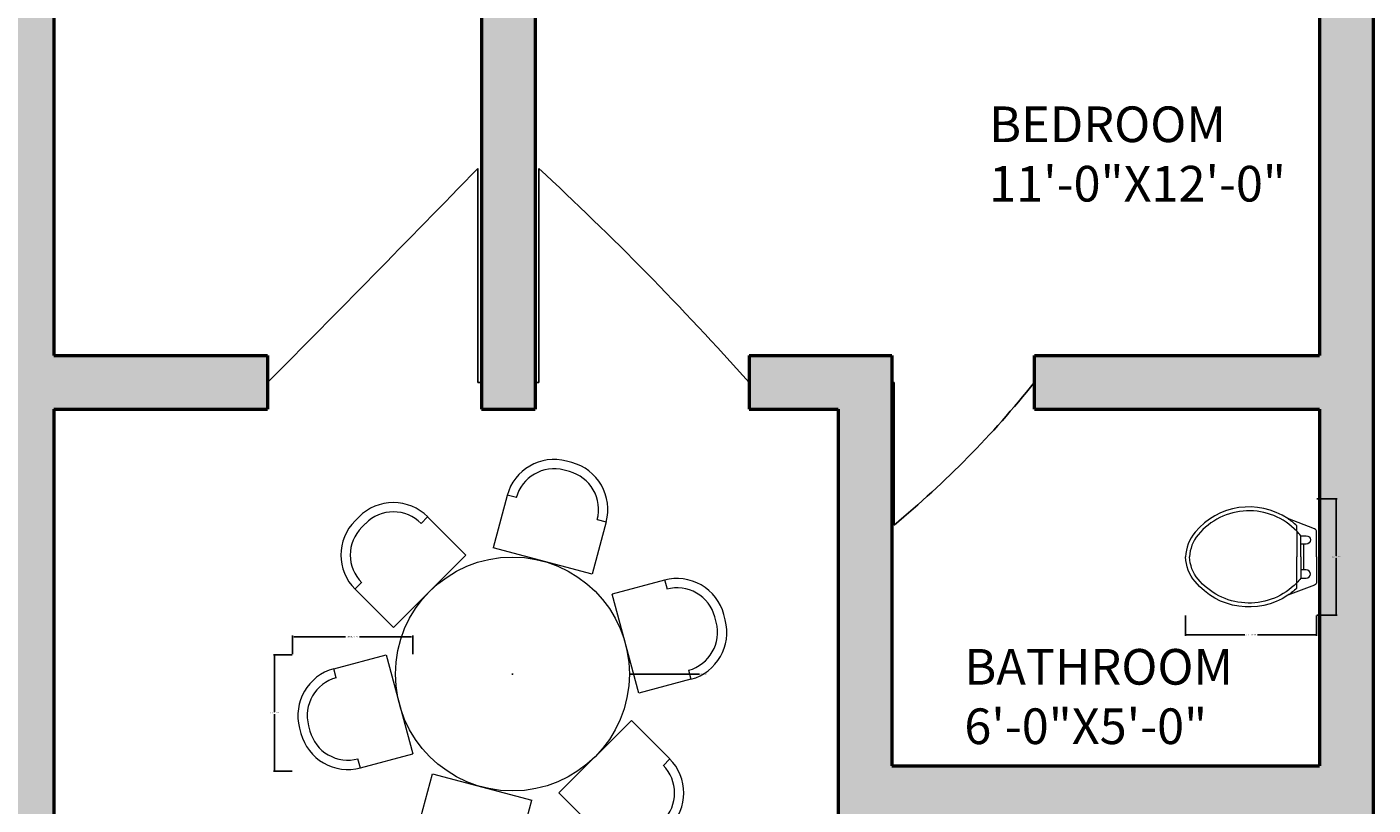
# Model space of a CAD drawing. Units: inches. Extents: x -17 to 536, y -817 to 53.
# Tile 8 of 9: x 268 to 494, y -217 to -86. Entities that reach past the tile are written whole.
import ezdxf

# ---------------------------------------------------------------- set-up
doc = ezdxf.new("R2010")
doc.units = ezdxf.units.IN
doc.header["$MEASUREMENT"] = 0
for name, color, linetype, lineweight in [('A-ANNO-DIMS', 2, 'Continuous', 18), ('A-AREA-IDEN', 7, 'Continuous', 18), ('A-DOOR', 4, 'Continuous', 25), ('A-FLOR-FIXT', 9, 'Continuous', 18), ('A-FURN', 8, 'Continuous', 13), ('A-WALL', 7, 'Continuous', 50), ('A-WALL-PATT', 22, 'Continuous', 13)]:
    doc.layers.add(name, color=color, linetype=linetype, lineweight=lineweight)
doc.styles.get("Standard").update_dxf_attribs({"font": 'arial.ttf'})
doc.dimstyles.get("Standard").update_dxf_attribs({"dimtxt": 0.18, "dimasz": 0.18, "dimexe": 0.18, "dimexo": 0.0625, "dimgap": 0.09, "dimtad": 0, "dimtih": 1, "dimtoh": 1, "dimdec": 0, "dimzin": 0, "dimdsep": 46, "dimlunit": 3, "dimtxsty": 'Standard', "dimcen": 0.09, "dimadec": 0, "dimazin": 0, "dimtfac": 1, "dimtdec": 0, "dimtofl": 0, "dimtmove": 0, "dimatfit": 3, "dimfxl": 1, "dimtolj": 1, "dimtzin": 0, "dimarcsym": 0})

# ---------------------------------------------------------------- blocks, each defined once
blk = doc.blocks.new('WC-22IN')
for p, q in [((18.71, 12.76), (18.71, 13.68)), ((18.71, 12.76), (18.71, 8.42)), ((18.71, 4.08), (18.71, 8.42)), ((18.71, 3.16), (18.71, 4.08))]:
    blk.add_line(p, q)
for points in [[(17.19, 14.88, 0.383919), (1.59, 12.57, 0.163732), (0, 8.42, 0.359733)], [(18.71, 12.76, 0.448546), (2.1, 12.15, 0.162618), (0.66, 8.42, 0.470877)], [(18.71, 13.68, 0.040937), (17.19, 14.88, 0.163732)], [(22.05, 8.42), (22.05, 12.63, 0.31031), (21.69, 13.15), (17.19, 14.88, 0.209071)], [(19.37, 12, 0.022712), (18.71, 12.76, 0.162618)], [(19.37, 8.42), (19.37, 12, 0.476108)], [(19.37, 12), (20.3, 12, -1), (20.3, 10.59), (19.82, 10.59)], [(17.19, 1.97, -0.383919), (1.59, 4.28, -0.163732), (0, 8.42, -0.359733)], [(18.26, 3.64, -0.431639), (2.1, 4.7, -0.162618), (0.66, 8.42, -0.470877)], [(22.05, 8.42), (22.05, 4.21, -0.31031), (21.69, 3.7), (17.19, 1.97, -0.209071)], [(19.37, 8.42), (19.37, 4.85, -0.022712)], [(19.37, 4.85, -0.022712), (18.71, 4.08, -0.162618)], [(19.37, 4.85), (20.3, 4.85, 1), (20.3, 6.25), (19.82, 6.25)], [(18.71, 3.16, -0.040937), (17.19, 1.97, -0.163732)], [(18.71, 4.08, -0.014165), (18.26, 3.64, -0.162618)]]:
    blk.add_lwpolyline(points, format="xyb")
for points in [[(19.82, 10.59), (19.37, 10.59)], [(19.82, 10.59), (19.82, 6.25)], [(19.82, 6.25), (19.37, 6.25)]]:
    blk.add_lwpolyline(points)
blk = doc.blocks.new('DINING-CHAIR-COMPACT')
for p, q in [((8.8, 19.04), (0, 16.68)), ((9.29, 17.47), (8.86, 19.06)), ((4.47, 0), (0, 16.68)), ((17.52, 11.95), (17.28, 12.86)), ((19.04, 12.35), (18.79, 13.26)), ((13.27, 2.36), (4.47, 0)), ((12.86, 3.87), (13.27, 2.36))]:
    blk.add_line(p, q)
for centre, radius, start, end in [((10.91, 11.15), 8.16, 15, 105), ((10.91, 11.15), 6.59, 15, 105), ((11.15, 10.24), 6.59, 285, 15), ((11.15, 10.24), 8.16, 285, 15)]:
    blk.add_arc(centre, radius, start, end)
blk = doc.blocks.new('*D16')
at = {"layer": 'A-ANNO-DIMS', "color": 0, "lineweight": -2, "transparency": 16777216}
for p, q in [((312.57, -191.71), (312.57, -188.56)), ((312.75, -188.74), (321.49, -188.74)), ((332.59, -188.74), (323.85, -188.74)), ((332.77, -191.71), (332.77, -188.56))]:
    blk.add_line(p, q, dxfattribs=at)
at = {"layer": 'A-ANNO-DIMS', "color": 0, "transparency": 16777216}
for points in [[(312.75, -188.71), (312.75, -188.77), (312.57, -188.74)], [(332.59, -188.71), (332.59, -188.77), (332.77, -188.74)]]:
    blk.add_solid(points, dxfattribs=at)
at = {"layer": 'Defpoints', "color": 0, "transparency": 16777216}
for p in [(312.57, -188.74), (312.57, -191.77), (332.77, -191.77)]:
    blk.add_point(p, dxfattribs=at)
at = {"layer": 'A-ANNO-DIMS', "color": 0, "transparency": 16777216, "insert": (322.67, -188.74), "char_height": 0.18, "attachment_point": 5}
blk.add_mtext('\\A1;CHAIR B 1\'-8" TYP.', dxfattribs=at)
blk = doc.blocks.new('*D17')
at = {"layer": 'A-ANNO-DIMS', "color": 0, "lineweight": -2, "transparency": 16777216}
for p, q in [((312.51, -191.77), (309.36, -191.77)), ((309.54, -191.95), (309.54, -201.39)), ((309.54, -211.19), (309.54, -201.75)), ((312.51, -211.37), (309.36, -211.37))]:
    blk.add_line(p, q, dxfattribs=at)
at = {"layer": 'A-ANNO-DIMS', "color": 0, "transparency": 16777216}
for points in [[(309.51, -191.95), (309.57, -191.95), (309.54, -191.77)], [(309.51, -211.19), (309.57, -211.19), (309.54, -211.37)]]:
    blk.add_solid(points, dxfattribs=at)
at = {"layer": 'Defpoints', "color": 0, "transparency": 16777216}
for p in [(312.57, -191.77), (309.54, -211.37), (312.57, -211.37)]:
    blk.add_point(p, dxfattribs=at)
at = {"layer": 'A-ANNO-DIMS', "color": 0, "transparency": 16777216, "insert": (309.54, -201.57), "char_height": 0.18, "attachment_point": 5}
blk.add_mtext('\\A1;1\'-7 1/2" TYP.', dxfattribs=at)
blk = doc.blocks.new('*D24')
at = {"layer": 'A-ANNO-DIMS', "color": 0, "lineweight": -2, "transparency": 16777216}
for p, q in [((462.82, -185.18), (462.82, -188.61)), ((484.87, -185.18), (484.87, -188.61)), ((463, -188.43), (472.77, -188.43)), ((484.69, -188.43), (474.92, -188.43))]:
    blk.add_line(p, q, dxfattribs=at)
at = {"layer": 'A-ANNO-DIMS', "color": 0, "transparency": 16777216}
for points in [[(463, -188.4), (463, -188.46), (462.82, -188.43)], [(484.69, -188.4), (484.69, -188.46), (484.87, -188.43)]]:
    blk.add_solid(points, dxfattribs=at)
at = {"layer": 'Defpoints', "color": 0, "transparency": 16777216}
for p in [(462.82, -185.12), (484.87, -185.12), (484.87, -188.43)]:
    blk.add_point(p, dxfattribs=at)
at = {"layer": 'A-ANNO-DIMS', "color": 0, "transparency": 16777216, "insert": (473.84, -188.43), "char_height": 0.18, "attachment_point": 5}
blk.add_mtext('\\A1;WC B 1\'-10" TYP.', dxfattribs=at)
blk = doc.blocks.new('*D25')
at = {"layer": 'A-ANNO-DIMS', "color": 0, "lineweight": -2, "transparency": 16777216}
for p, q in [((484.93, -165.53), (488.35, -165.53)), ((488.17, -165.71), (488.17, -175.14)), ((488.17, -184.94), (488.17, -175.51)), ((484.93, -185.12), (488.35, -185.12))]:
    blk.add_line(p, q, dxfattribs=at)
at = {"layer": 'A-ANNO-DIMS', "color": 0, "transparency": 16777216}
for points in [[(488.14, -165.71), (488.2, -165.71), (488.17, -165.53)], [(488.14, -184.94), (488.2, -184.94), (488.17, -185.12)]]:
    blk.add_solid(points, dxfattribs=at)
at = {"layer": 'Defpoints', "color": 0, "transparency": 16777216}
for p in [(484.87, -165.53), (488.17, -165.53), (484.87, -185.12)]:
    blk.add_point(p, dxfattribs=at)
at = {"layer": 'A-ANNO-DIMS', "color": 0, "transparency": 16777216, "insert": (488.17, -175.33), "char_height": 0.18, "attachment_point": 5}
blk.add_mtext('\\A1;1\'-7 1/2" TYP.', dxfattribs=at)
blk = doc.blocks.new('*D44')
at = {"layer": 'A-ANNO-DIMS', "color": 0, "lineweight": -2, "transparency": 16777216}
for p, q in [((349.46, -195.02), (349.64, -195.02)), ((349.55, -195.11), (349.55, -194.93)), ((381.04, -195.02), (369.41, -195.02))]:
    blk.add_line(p, q, dxfattribs=at)
at = {"layer": 'A-ANNO-DIMS', "color": 0, "transparency": 16777216}
blk.add_solid([(369.41, -194.99), (369.41, -195.05), (369.23, -195.02)], dxfattribs=at)
at = {"layer": 'Defpoints', "color": 0, "transparency": 16777216}
for p in [(329.87, -195.02), (369.23, -195.02)]:
    blk.add_point(p, dxfattribs=at)
at = {"layer": 'A-ANNO-DIMS', "color": 0, "transparency": 16777216, "insert": (381.68, -195.02), "char_height": 0.18, "attachment_point": 5}
blk.add_mtext('\\A1;∅3\'-3 1/2"', dxfattribs=at)

msp = doc.modelspace()

# ---------------------------------------------------------------- hatches: boundary and pattern name
at = {"layer": 'A-WALL-PATT'}
h = msp.add_hatch(color=256, dxfattribs=at)
h.dxf.hatch_style = 1
h.paths.add_polyline_path([(217.37, -544.45), (208.37, -544.45), (208.37, -775.45), (217.37, -775.45)], flags=17)
h.paths.add_polyline_path([(327.37, -544.45), (318.37, -544.45), (318.37, -775.45), (327.37, -775.45)], flags=17)
h.paths.add_polyline_path([(494.37, 11.55), (41.37, 11.55), (41.37, -775.45), (50.37, -775.45), (50.37, -739.45), (184.37, -739.45), (184.37, -730.45), (50.37, -730.45), (50.37, -610.45), (172.37, -610.45), (172.37, -601.45), (155.37, -601.45), (155.37, -577.45), (146.37, -577.45), (146.37, -601.45), (50.37, -601.45), (50.37, -553.45), (172.37, -553.45), (172.37, -544.45), (50.37, -544.45), (50.37, -436.45), (191.37, -436.45), (191.37, -319.45), (182.37, -319.45), (182.37, -427.45), (50.37, -427.45), (50.37, -283.45), (98.37, -283.45), (98.37, -274.45), (50.37, -274.45), (50.37, -219.45), (122.37, -219.45), (122.37, -283.45), (191.37, -283.45), (191.37, -274.45), (131.37, -274.45), (131.37, -219.45), (131.37, -150.45), (146.37, -150.45), (146.37, -141.45), (122.37, -141.45), (122.37, -210.45), (50.37, -210.45), (50.37, -150.45), (98.37, -150.45), (98.37, -141.45), (50.37, -141.45), (50.37, 2.55), (182.37, 2.55), (182.37, -150.45), (191.37, -150.45), (191.37, 2.55), (263.37, 2.55), (263.37, -141.45), (227.37, -141.45), (227.37, -150.45), (263.37, -150.45), (263.37, -553.45), (272.37, -553.45), (272.37, -150.45), (308.37, -150.45), (308.37, -141.45), (272.37, -141.45), (272.37, 2.55), (344.37, 2.55), (344.37, -150.45), (353.37, -150.45), (353.37, 2.55), (485.37, 2.55), (485.37, -141.45), (437.37, -141.45), (437.37, -150.45), (485.37, -150.45), (485.37, -210.45), (413.37, -210.45), (413.37, -141.45), (389.37, -141.45), (389.37, -150.45), (404.37, -150.45), (404.37, -219.45), (404.37, -274.45), (353.37, -274.45), (344.37, -274.45), (344.37, -283.45), (353.37, -283.45), (413.37, -283.45), (413.37, -219.45), (485.37, -219.45), (485.37, -274.45), (437.37, -274.45), (437.37, -283.45), (485.37, -283.45), (485.37, -427.45), (353.37, -427.45), (353.37, -319.45), (344.37, -319.45), (344.37, -436.45), (485.37, -436.45), (485.37, -544.45), (363.37, -544.45), (363.37, -553.45), (485.37, -553.45), (485.37, -601.45), (389.37, -601.45), (389.37, -577.45), (380.37, -577.45), (380.37, -601.45), (363.37, -601.45), (363.37, -610.45), (485.37, -610.45), (485.37, -730.45), (351.37, -730.45), (351.37, -739.45), (485.37, -739.45), (485.37, -775.45), (494.37, -775.45)])

# ---------------------------------------------------------------- linework, layer by layer
at = {"layer": 'A-DOOR'}
for p, q in [((343.72, -145.95), (343.72, -109.95)), ((353.99, -145.95), (353.99, -109.95)), ((343.72, -145.95), (344.37, -145.95)), ((353.99, -145.95), (353.37, -145.95)), ((413.77, -145.95), (413.37, -145.95)), ((413.77, -145.95), (413.77, -169.95))]:
    msp.add_line(p, q, dxfattribs=at)
for centre, radius, start, end in [((-3120.49, 3256.59), 4830.57, 315.2207, 315.81916), ((-4.63, -497.73), 528.19, 41.7601, 47.2371), ((309.76, -44.1), 163.27, 309.5739, 321.4053)]:
    msp.add_arc(centre, radius, start, end, dxfattribs=at)
at = {"layer": 'A-FURN'}
msp.add_circle((349.55, -195.02), 19.68, dxfattribs=at)
at = {"layer": 'A-WALL'}
for p, q in [((494.37, 11.55), (494.37, -775.45)), ((272.37, 2.55), (272.37, -141.45)), ((344.37, 2.55), (344.37, -150.45)), ((353.37, 2.55), (353.37, -150.45)), ((485.37, 2.55), (485.37, -141.45)), ((272.37, -141.45), (308.37, -141.45)), ((308.37, -141.45), (308.37, -150.45)), ((389.37, -141.45), (413.37, -141.45)), ((389.37, -141.45), (389.37, -150.45)), ((413.37, -141.45), (413.37, -210.45)), ((437.37, -150.45), (437.37, -141.45)), ((437.37, -141.45), (485.37, -141.45)), ((272.37, -150.45), (308.37, -150.45)), ((272.37, -150.45), (272.37, -553.45)), ((344.37, -150.45), (353.37, -150.45)), ((389.37, -150.45), (404.37, -150.45)), ((404.37, -150.45), (404.37, -219.45)), ((437.37, -150.45), (485.37, -150.45)), ((485.37, -150.45), (485.37, -210.45)), ((413.37, -210.45), (485.37, -210.45))]:
    msp.add_line(p, q, dxfattribs=at)

# ---------------------------------------------------------------- block references
at = {"layer": 'A-FLOR-FIXT'}
msp.add_blockref('WC-22IN', (462.82, -183.75), dxfattribs=at)
at = {"layer": 'A-FURN'}
for p, rotation in [((360.75, -182.11), 59.99999997356139), ((343.97, -178.87), 120.0000000057714), ((332.77, -191.77), 180), ((355.13, -211.17), 300.0000000082552), ((338.35, -207.92), 239.999999980094)]:
    msp.add_blockref('DINING-CHAIR-COMPACT', p, dxfattribs=dict(at, rotation=rotation))
msp.add_blockref('DINING-CHAIR-COMPACT', (366.33, -198.26), dxfattribs=at)

# ---------------------------------------------------------------- texts
at = {"layer": 'A-AREA-IDEN', "char_height": 6, "attachment_point": 1}
for s, insert in [('BEDROOM\\P11\'-0"X12\'-0"', (429.77, -99.52)), ('BATHROOM\\P6\'-0"X5\'-0"', (425.59, -190.81))]:
    msp.add_mtext(s, dxfattribs=dict(at, insert=insert))

# ---------------------------------------------------------------- dimensions: what is measured, and where the dimension line sits
at = {"layer": 'A-ANNO-DIMS'}
for base, p1, p2, angle, text, picture, middle in [((488.17, -165.53), (484.87, -185.12), (484.87, -165.53), 90, '<> TYP.', '*D25', (488.17, -175.33)), ((312.57, -188.74), (332.77, -191.77), (312.57, -191.77), 180, 'CHAIR B <> TYP.', '*D16', (322.67, -188.74)), ((309.54, -211.37), (312.57, -191.77), (312.57, -211.37), 270, '<> TYP.', '*D17', (309.54, -201.57))]:
    dim = msp.add_linear_dim(base=base, p1=p1, p2=p2, angle=angle, text=text, dimstyle='Standard', override={"dimdec": 1, "dimlfac": 1, "dimrnd": 0, "dimzin": 1, "dimdsep": 46, "dimlunit": 4, "dimfrac": 2}, dxfattribs=at)
    dim.commit()
    dim.dimension.update_dxf_attribs({"geometry": picture, "text_midpoint": middle})
dim = msp.add_linear_dim(base=(484.865, -188.4267), p1=(462.8197, -185.1199), p2=(484.865, -185.1199), text='WC B <> TYP.', dimstyle='Standard', override={"dimdec": 1, "dimlfac": 1, "dimrnd": 0, "dimzin": 1, "dimdsep": 46, "dimlunit": 4, "dimfrac": 2}, dxfattribs=at)
dim.commit()
dim.dimension.update_dxf_attribs({"geometry": '*D24', "text_midpoint": (473.8424, -188.4267)})
dim = msp.add_diameter_dim_2p(p1=(329.87, -195.02), p2=(369.23, -195.02), dimstyle='Standard', override={"dimdec": 1, "dimlfac": 1, "dimrnd": 0, "dimzin": 1, "dimdsep": 46, "dimlunit": 4, "dimfrac": 2}, dxfattribs=at)
dim.commit()
dim.dimension.update_dxf_attribs({"geometry": '*D44', "text_midpoint": (381.04, -195.02), "dimtype": 163})

doc.saveas('drawing.dxf')
